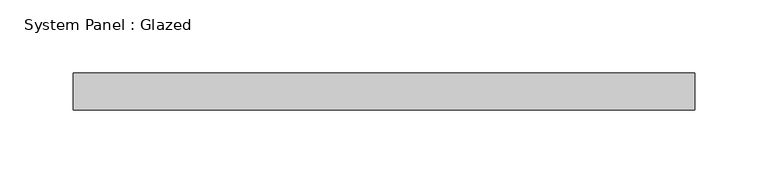
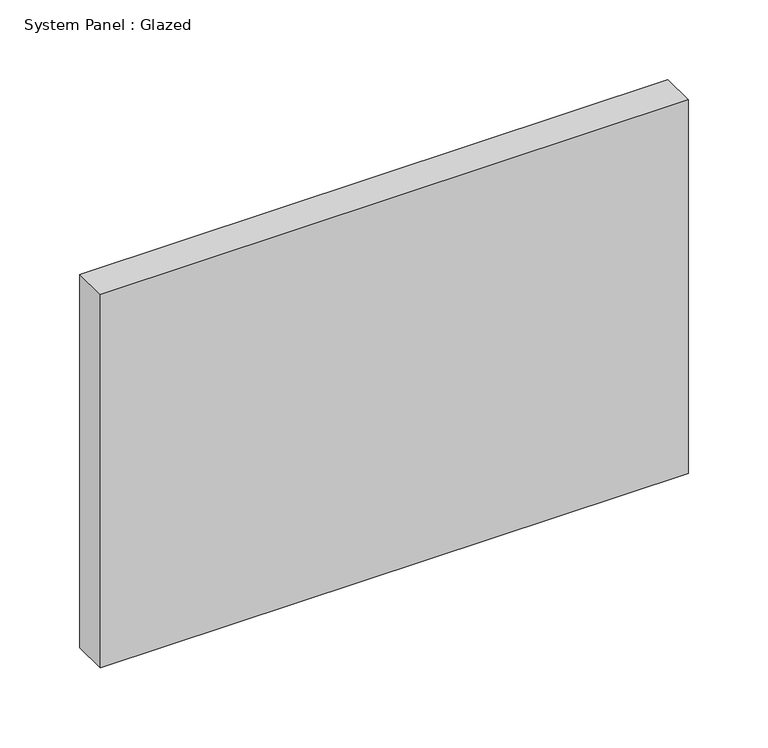
"""IFC4 building model written with IfcOpenShell, lengths in millimetres: plate geometry, System Panel : Glazed."""

from ifc_helpers import new_model, si_unit, origin, origin_with_axes, place, context, project, spatial, polyline, outline, extrude, source, transform, mapped, element, save


def system_panel_glazed_73771f90(model_context):
    return source(origin(), model_context, "Body", "SweptSolid", [
        extrude(outline(polyline([(212.725, 19.05), (-212.725, 19.05), (-212.725, 44.45), (212.725, 44.45), (212.725, 19.05)])), origin_with_axes(), (0.0, 0.0, 1.0), 285.75),
    ])


if __name__ == "__main__":
    model = new_model("IFC4")
    model_context = context("Model", 3, world=origin())
    ifc_project = project(units=[si_unit("LENGTHUNIT", "METRE", prefix="MILLI")], contexts=[model_context])
    site = spatial("IfcSite", under=ifc_project)
    building = spatial("IfcBuilding", under=site)
    placement = place(None, origin())
    system_panel_glazed_shape = system_panel_glazed_73771f90(model_context)
    element("IfcPlate", 1, ObjectType="System Panel : Glazed", at=placement, inside=building, context=model_context, shape_type="MappedRepresentation", body=[
        mapped(system_panel_glazed_shape, transform((0.0, 0.0, 0.0), x_axis=(1.0, 0.0, 0.0), y_axis=(0.0, 1.0, 0.0), z_axis=(0.0, 0.0, 1.0))),
    ])
    save(model, "model.ifc")

# Revit data of these elements
# Type "System Panel : Glazed"
#   Construction Type Id = "GSP4R"
#   Analytic Construction = "1/8 in Pilkington single glazing"
#   Visual Light Transmittance = 0.9
#   Solar Heat Gain Coefficient = 0.86
#   Heat Transfer Coefficient (U) = 1.18115 BTU/(h·ft²·°F)
#   Define Thermal Properties by = 1
# Element 1 (IfcPlate, "System Panel : Glazed")
#   Materials on its faces: "Glass"
# Materials
#   "Glass": class "Glass", colour RGB 0 128 192, transparency 0.75, Description = "Soda Lime Glass", Cost = 0
